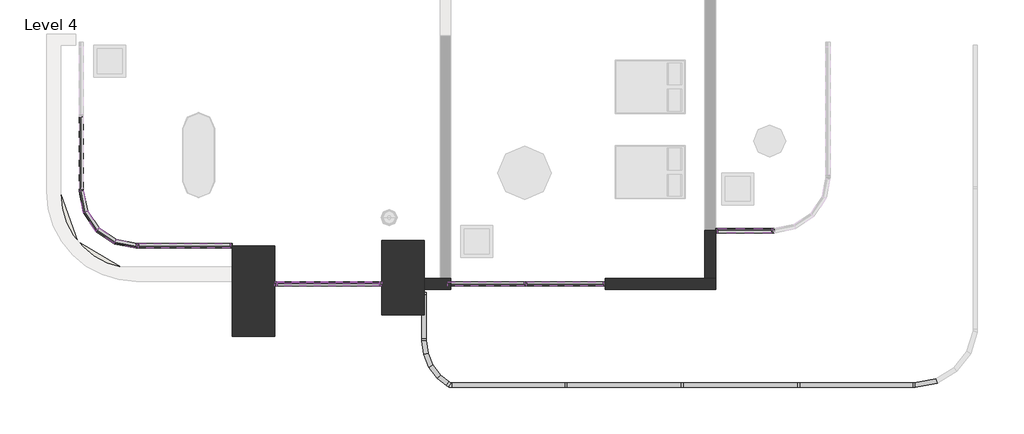
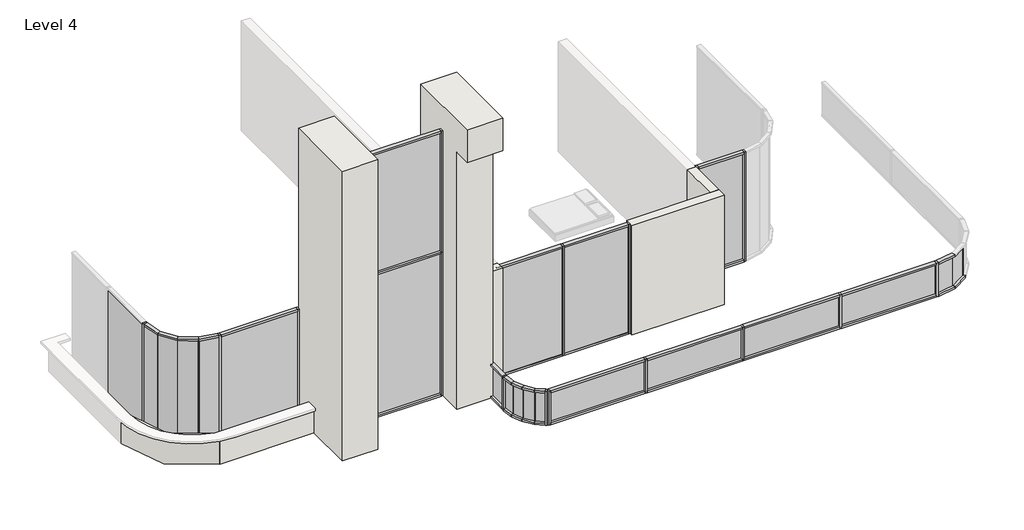
# One storey, part 1 of 2: 61 members, 22 plates, 7 walls.
"""IFC4 building model written with IfcOpenShell, lengths in millimetres."""

from ifc_helpers import new_model, si_unit, point, frame, frame_2d, origin, place, context, project, spatial, polyline, circle_curve, trimmed, segment, composite_curve, outline, extrude, faceted_brep, transform, mapped, element, save
from components import member_e5c989f4, member_5be86ab4, member_8daf8b49, member_d457d5cf, member_70c1698b, member_c6c1cc64, member_2ed7bf35, member_fedd83b6, member_820ab859, member_e6e8f276, member_9bbfae49, member_71eb4692, member_3c8bcf7e, member_dede372a, member_2b49869a, member_75074519, member_068c4367, member_d18c953d, member_1e511d5c, member_f1972444, member_37af120a, member_fe018dc2, member_83685764, member_73d0c9ee, member_70a47126, member_8f078878, system_panel_glazed_da3fd9d5, system_panel_glazed_e9252991, system_panel_glazed_d7bd2e6f, system_panel_glazed_62c681ce, system_panel_glazed_5d8041e7, system_panel_glazed_8818662e, system_panel_glazed_df7f3c5e, system_panel_glazed_53e0be6b, system_panel_glazed_e0d10779, system_panel_glazed_9262d402, system_panel_glazed_b9e36109, system_panel_glazed_ffaa535b, system_panel_glazed_1f819173

model = new_model("IFC4")

# Units and contexts
model_context = context("Model", 3, world=origin())
ifc_project = project(units=[si_unit("LENGTHUNIT", "METRE", prefix="MILLI")], contexts=[model_context])

# Site, building, storey
site = spatial("IfcSite", under=ifc_project)
building = spatial("IfcBuilding", under=site)
storey = spatial("IfcBuildingStorey", under=building, Name="Level 4", Elevation=6096.0)

# Members
placement = place(None, origin())
member_shape = member_e5c989f4(model_context)
element("IfcMember", 1, ObjectType="Rectangular Mullion : 2.5\" x 5\" rectangular", at=placement, inside=storey, context=model_context, shape_type="MappedRepresentation", body=[
    mapped(member_shape, transform((-4022.036879, -4118.7908042, 5994.4), x_axis=(-1.0, 0.0, 0.0), y_axis=(0.0, 1.0, 0.0), z_axis=(0.0, 0.0, -1.0))),
])
member_2_shape = member_5be86ab4(model_context)
element("IfcMember", 2, ObjectType="Rectangular Mullion : 2.5\" x 5\" rectangular", at=placement, inside=storey, context=model_context, shape_type="MappedRepresentation", body=[
    mapped(member_2_shape, transform((-6308.036879, -4118.7908042, 5994.4), x_axis=(-1.0, 0.0, 0.0), y_axis=(0.0, 1.0, 0.0), z_axis=(0.0, 0.0, -1.0))),
])
element("IfcMember", 3, ObjectType="Rectangular Mullion : 2.5\" x 5\" rectangular", at=placement, inside=storey, context=model_context, shape_type="MappedRepresentation", body=[
    mapped(member_2_shape, transform((3089.963121, -2594.7908042, 5994.4), x_axis=(1.0, 0.0, 0.0), y_axis=(0.0, -1.0, 0.0), z_axis=(0.0, 0.0, -1.0))),
])
element("IfcMember", 4, ObjectType="Rectangular Mullion : 2.5\" x 5\" rectangular", at=placement, inside=storey, context=model_context, shape_type="MappedRepresentation", body=[
    mapped(member_2_shape, transform((-15147.236879, -3028.3602909, 5994.4), x_axis=(-1.0, 0.0, 0.0), y_axis=(0.0, 1.0, 0.0), z_axis=(0.0, 0.0, -1.0))),
])
element("IfcMember", 5, ObjectType="Rectangular Mullion : 2.5\" x 5\" rectangular", at=placement, inside=storey, context=model_context, shape_type="MappedRepresentation", body=[
    mapped(member_2_shape, transform((-1736.036879, -4118.7908042, 9956.8), x_axis=(1.0, 0.0, 0.0), y_axis=(0.0, 1.0, 0.0), z_axis=(0.0, 0.0, 1.0))),
])
element("IfcMember", 6, ObjectType="Rectangular Mullion : 2.5\" x 5\" rectangular", at=placement, inside=storey, context=model_context, shape_type="MappedRepresentation", body=[
    mapped(member_2_shape, transform((1413.563121, -2594.7908042, 9956.8), x_axis=(-1.0, 0.0, 0.0), y_axis=(0.0, -1.0, 0.0), z_axis=(0.0, 0.0, 1.0))),
])
element("IfcMember", 7, ObjectType="Rectangular Mullion : 2.5\" x 5\" rectangular", at=placement, inside=storey, context=model_context, shape_type="MappedRepresentation", body=[
    mapped(member_2_shape, transform((-12404.036879, -3028.3602909, 9956.8), x_axis=(1.0, 0.0, 0.0), y_axis=(0.0, 1.0, 0.0), z_axis=(0.0, 0.0, 1.0))),
])
element("IfcMember", 8, ObjectType="Rectangular Mullion : 2.5\" x 5\" rectangular", at=placement, inside=storey, context=model_context, shape_type="MappedRepresentation", body=[
    mapped(member_2_shape, transform((-16724.4155088, -1451.181661, 9956.8), x_axis=(0.0, -1.0, 0.0), y_axis=(1.0, 0.0, 0.0), z_axis=(0.0, 0.0, 1.0))),
])
member_3_shape = member_8daf8b49(model_context)
element("IfcMember", 9, ObjectType="Rectangular Mullion : 2.5\" x 5\" rectangular", at=placement, inside=storey, context=model_context, shape_type="MappedRepresentation", body=[
    mapped(member_3_shape, transform((-6244.536879, -4118.7908042, 9956.8), x_axis=(0.0, 0.0, 1.0), y_axis=(0.0, 1.0, 0.0), z_axis=(-1.0, 0.0, 0.0))),
])
element("IfcMember", 10, ObjectType="Rectangular Mullion : 2.5\" x 5\" rectangular", at=placement, inside=storey, context=model_context, shape_type="MappedRepresentation", body=[
    mapped(member_3_shape, transform((-3990.286879, -4118.7908042, 9956.8), x_axis=(0.0, 0.0, 1.0), y_axis=(0.0, 1.0, 0.0), z_axis=(-1.0, 0.0, 0.0))),
])
element("IfcMember", 11, ObjectType="Rectangular Mullion : 2.5\" x 5\" rectangular", at=placement, inside=storey, context=model_context, shape_type="MappedRepresentation", body=[
    mapped(member_3_shape, transform((-1799.536879, -4118.7908042, 5994.4), x_axis=(0.0, 0.0, -1.0), y_axis=(0.0, 1.0, 0.0), z_axis=(1.0, 0.0, 0.0))),
])
element("IfcMember", 12, ObjectType="Rectangular Mullion : 2.5\" x 5\" rectangular", at=placement, inside=storey, context=model_context, shape_type="MappedRepresentation", body=[
    mapped(member_3_shape, transform((-4053.786879, -4118.7908042, 5994.4), x_axis=(0.0, 0.0, -1.0), y_axis=(0.0, 1.0, 0.0), z_axis=(1.0, 0.0, 0.0))),
])
member_4_shape = member_d457d5cf(model_context)
element("IfcMember", 13, ObjectType="Rectangular Mullion : 2.5\" x 5\" rectangular", at=placement, inside=storey, context=model_context, shape_type="MappedRepresentation", body=[
    mapped(member_4_shape, transform((-8200.336879, -4118.7908042, 15572.5549749), x_axis=(0.0, 0.0, 1.0), y_axis=(0.0, -1.0, 0.0), z_axis=(1.0, 0.0, 0.0))),
])
element("IfcMember", 14, ObjectType="Rectangular Mullion : 2.5\" x 5\" rectangular", at=placement, inside=storey, context=model_context, shape_type="MappedRepresentation", body=[
    mapped(member_4_shape, transform((-11121.336879, -4118.7908042, 5994.4), x_axis=(0.0, 0.0, -1.0), y_axis=(0.0, -1.0, 0.0), z_axis=(-1.0, 0.0, 0.0))),
])
member_5_shape = member_70c1698b(model_context)
element("IfcMember", 15, ObjectType="Rectangular Mullion : 2.5\" x 5\" rectangular", at=placement, inside=storey, context=model_context, shape_type="MappedRepresentation", body=[
    mapped(member_5_shape, transform((-15083.736879, -3028.3602909, 9956.8), x_axis=(0.0, 0.0, 1.0), y_axis=(0.0, 1.0, 0.0), z_axis=(-1.0, 0.0, 0.0))),
])
element("IfcMember", 16, ObjectType="Rectangular Mullion : 2.5\" x 5\" rectangular", at=placement, inside=storey, context=model_context, shape_type="MappedRepresentation", body=[
    mapped(member_5_shape, transform((-12467.536879, -3028.3602909, 5994.4), x_axis=(0.0, 0.0, -1.0), y_axis=(0.0, 1.0, 0.0), z_axis=(1.0, 0.0, 0.0))),
])
member_6_shape = member_c6c1cc64(model_context)
element("IfcMember", 17, ObjectType="Rectangular Mullion : 2.5\" x 5\" rectangular", at=placement, inside=storey, context=model_context, shape_type="MappedRepresentation", body=[
    mapped(member_6_shape, transform((-16262.4705833, -2566.4153653, 9956.8), x_axis=(0.0, 0.0, 1.0), y_axis=(0.5555702330196196, 0.8314696123025338, 0.0), z_axis=(-0.8314696123025338, 0.5555702330196196, 0.0))),
])
element("IfcMember", 18, ObjectType="Rectangular Mullion : 2.5\" x 5\" rectangular", at=placement, inside=storey, context=model_context, shape_type="MappedRepresentation", body=[
    mapped(member_6_shape, transform((-15750.7970105, -2908.3047162, 5994.4), x_axis=(0.0, 0.0, -1.0), y_axis=(0.5555702330196196, 0.8314696123025338, 0.0), z_axis=(0.8314696123025338, -0.5555702330196196, 0.0))),
])
element("IfcMember", 19, ObjectType="Rectangular Mullion : 2.5\" x 5\" rectangular", at=placement, inside=storey, context=model_context, shape_type="MappedRepresentation", body=[
    mapped(member_6_shape, transform((-16262.4705833, -2566.4153653, 5994.4), x_axis=(0.0, 0.0, -1.0), y_axis=(0.831469612302556, 0.5555702330195863, 0.0), z_axis=(0.5555702330195863, -0.831469612302556, 0.0))),
])
element("IfcMember", 20, ObjectType="Rectangular Mullion : 2.5\" x 5\" rectangular", at=placement, inside=storey, context=model_context, shape_type="MappedRepresentation", body=[
    mapped(member_6_shape, transform((-16604.3599342, -2054.7417925, 9956.8), x_axis=(0.0, 0.0, 1.0), y_axis=(0.8314696123025557, 0.5555702330195866, 0.0), z_axis=(-0.5555702330195866, 0.8314696123025557, 0.0))),
])
member_7_shape = member_2ed7bf35(model_context)
element("IfcMember", 21, ObjectType="Rectangular Mullion : 2.5\" x 5\" rectangular", at=placement, inside=storey, context=model_context, shape_type="MappedRepresentation", body=[
    mapped(member_7_shape, transform((-8200.336879, -4118.7908042, 11176.0), x_axis=(0.0, 0.0, 1.0), y_axis=(0.0, -1.0, 0.0), z_axis=(1.0, 0.0, 0.0))),
])
member_8_shape = member_fedd83b6(model_context)
element("IfcMember", 22, ObjectType="Rectangular Mullion : 2.5\" x 5\" rectangular", at=placement, inside=storey, context=model_context, shape_type="MappedRepresentation", body=[
    mapped(member_8_shape, transform((3026.463121, -2594.7908042, 9956.8), x_axis=(0.0, 0.0, 1.0), y_axis=(0.0, -1.0, 0.0), z_axis=(1.0, 0.0, 0.0))),
])
element("IfcMember", 23, ObjectType="Rectangular Mullion : 2.5\" x 5\" rectangular", at=placement, inside=storey, context=model_context, shape_type="MappedRepresentation", body=[
    mapped(member_8_shape, transform((1477.063121, -2594.7908042, 5994.4), x_axis=(0.0, 0.0, -1.0), y_axis=(0.0, -1.0, 0.0), z_axis=(-1.0, 0.0, 0.0))),
])
member_9_shape = member_820ab859(model_context)
element("IfcMember", 24, ObjectType="Rectangular Mullion : 2.5\" x 5\" rectangular", at=placement, inside=storey, context=model_context, shape_type="MappedRepresentation", body=[
    mapped(member_9_shape, transform((-16724.4155088, -1387.681661, 5994.4), x_axis=(0.0, 0.0, -1.0), y_axis=(1.0, 0.0, 0.0), z_axis=(0.0, -1.0, 0.0))),
])
member_10_shape = member_e6e8f276(model_context)
element("IfcMember", 25, ObjectType="Rectangular Mullion : 2.5\" x 5\" rectangular", at=placement, inside=storey, context=model_context, shape_type="MappedRepresentation", body=[
    mapped(member_10_shape, transform((-15147.236879, -3028.3602909, 5994.4), x_axis=(0.0, 0.0, -1.0), y_axis=(0.19509032201614443, 0.9807852804032272, 0.0), z_axis=(0.9807852804032271, -0.1950903220161444, 0.0))),
])
member_11_shape = member_9bbfae49(model_context)
element("IfcMember", 26, ObjectType="Rectangular Mullion : 2.5\" x 5\" rectangular", at=placement, inside=storey, context=model_context, shape_type="MappedRepresentation", body=[
    mapped(member_11_shape, transform((-15750.7970105, -2908.3047162, 9956.8), x_axis=(0.0, 0.0, 1.0), y_axis=(0.19509032201614443, 0.9807852804032272, 0.0), z_axis=(-0.9807852804032271, 0.1950903220161444, 0.0))),
])
element("IfcMember", 27, ObjectType="Rectangular Mullion : 2.5\" x 5\" rectangular", at=placement, inside=storey, context=model_context, shape_type="MappedRepresentation", body=[
    mapped(member_10_shape, transform((-16724.4155088, -1451.181661, 9956.8), x_axis=(0.0, 0.0, 1.0), y_axis=(0.9807852804032322, 0.1950903220161199, 0.0), z_axis=(-0.1950903220161199, 0.9807852804032322, 0.0))),
])
element("IfcMember", 28, ObjectType="Rectangular Mullion : 2.5\" x 5\" rectangular", at=placement, inside=storey, context=model_context, shape_type="MappedRepresentation", body=[
    mapped(member_11_shape, transform((-16604.3599342, -2054.7417925, 5994.4), x_axis=(0.0, 0.0, -1.0), y_axis=(0.9807852804032322, 0.1950903220161199, 0.0), z_axis=(0.1950903220161199, -0.9807852804032322, 0.0))),
])
member_12_shape = member_71eb4692(model_context)
element("IfcMember", 29, ObjectType="Rectangular Mullion : 2.5\" x 5\" rectangular", at=placement, inside=storey, context=model_context, shape_type="MappedRepresentation", body=[
    mapped(member_12_shape, transform((-6917.636879, -5676.9, 7213.6), x_axis=(0.0, 0.0, 1.0), y_axis=(-1.0, 0.0, 0.0), z_axis=(0.0, -1.0, 0.0))),
])
element("IfcMember", 30, ObjectType="Rectangular Mullion : 2.5\" x 5\" rectangular", at=placement, inside=storey, context=model_context, shape_type="MappedRepresentation", body=[
    mapped(member_12_shape, transform((-6917.636879, -4432.3, 5994.4), x_axis=(0.0, 0.0, -1.0), y_axis=(-1.0, 0.0, 0.0), z_axis=(0.0, 1.0, 0.0))),
])
member_13_shape = member_3c8bcf7e(model_context)
element("IfcMember", 31, ObjectType="Rectangular Mullion : 2.5\" x 5\" rectangular", at=placement, inside=storey, context=model_context, shape_type="MappedRepresentation", body=[
    mapped(member_13_shape, transform((7048.5, -7010.4, 7213.6), x_axis=(0.0, 0.0, 1.0), y_axis=(0.0, -1.0, 0.0), z_axis=(1.0, 0.0, 0.0))),
])
element("IfcMember", 32, ObjectType="Rectangular Mullion : 2.5\" x 5\" rectangular", at=placement, inside=storey, context=model_context, shape_type="MappedRepresentation", body=[
    mapped(member_13_shape, transform((-2901.95, -7010.4, 7213.6), x_axis=(0.0, 0.0, 1.0), y_axis=(0.0, -1.0, 0.0), z_axis=(1.0, 0.0, 0.0))),
])
member_14_shape = member_dede372a(model_context)
element("IfcMember", 33, ObjectType="Rectangular Mullion : 2.5\" x 5\" rectangular", at=placement, inside=storey, context=model_context, shape_type="MappedRepresentation", body=[
    mapped(member_14_shape, transform((425.45, -7010.4, 7213.6), x_axis=(0.0, 0.0, 1.0), y_axis=(0.0, -1.0, 0.0), z_axis=(1.0, 0.0, 0.0))),
])
element("IfcMember", 34, ObjectType="Rectangular Mullion : 2.5\" x 5\" rectangular", at=placement, inside=storey, context=model_context, shape_type="MappedRepresentation", body=[
    mapped(member_14_shape, transform((3752.85, -7010.4, 7213.6), x_axis=(0.0, 0.0, 1.0), y_axis=(0.0, -1.0, 0.0), z_axis=(1.0, 0.0, 0.0))),
])
element("IfcMember", 35, ObjectType="Rectangular Mullion : 2.5\" x 5\" rectangular", at=placement, inside=storey, context=model_context, shape_type="MappedRepresentation", body=[
    mapped(member_13_shape, transform((-6134.1, -7010.4, 5994.4), x_axis=(0.0, 0.0, -1.0), y_axis=(0.0, -1.0, 0.0), z_axis=(-1.0, 0.0, 0.0))),
])
element("IfcMember", 36, ObjectType="Rectangular Mullion : 2.5\" x 5\" rectangular", at=placement, inside=storey, context=model_context, shape_type="MappedRepresentation", body=[
    mapped(member_13_shape, transform((3816.35, -7010.4, 5994.4), x_axis=(0.0, 0.0, -1.0), y_axis=(0.0, -1.0, 0.0), z_axis=(-1.0, 0.0, 0.0))),
])
element("IfcMember", 37, ObjectType="Rectangular Mullion : 2.5\" x 5\" rectangular", at=placement, inside=storey, context=model_context, shape_type="MappedRepresentation", body=[
    mapped(member_14_shape, transform((-2838.45, -7010.4, 5994.4), x_axis=(0.0, 0.0, -1.0), y_axis=(0.0, -1.0, 0.0), z_axis=(-1.0, 0.0, 0.0))),
])
element("IfcMember", 38, ObjectType="Rectangular Mullion : 2.5\" x 5\" rectangular", at=placement, inside=storey, context=model_context, shape_type="MappedRepresentation", body=[
    mapped(member_14_shape, transform((488.95, -7010.4, 5994.4), x_axis=(0.0, 0.0, -1.0), y_axis=(0.0, -1.0, 0.0), z_axis=(-1.0, 0.0, 0.0))),
])
member_15_shape = member_2b49869a(model_context)
element("IfcMember", 39, ObjectType="Rectangular Mullion : 2.5\" x 5\" rectangular", at=placement, inside=storey, context=model_context, shape_type="MappedRepresentation", body=[
    mapped(member_15_shape, transform((-2870.2, -7010.4, 5994.4), x_axis=(1.0, 0.0, 0.0), y_axis=(0.0, -1.0, 0.0), z_axis=(0.0, 0.0, -1.0))),
])
element("IfcMember", 40, ObjectType="Rectangular Mullion : 2.5\" x 5\" rectangular", at=placement, inside=storey, context=model_context, shape_type="MappedRepresentation", body=[
    mapped(member_15_shape, transform((457.2, -7010.4, 5994.4), x_axis=(1.0, 0.0, 0.0), y_axis=(0.0, -1.0, 0.0), z_axis=(0.0, 0.0, -1.0))),
])
element("IfcMember", 41, ObjectType="Rectangular Mullion : 2.5\" x 5\" rectangular", at=placement, inside=storey, context=model_context, shape_type="MappedRepresentation", body=[
    mapped(member_15_shape, transform((3784.6, -7010.4, 5994.4), x_axis=(1.0, 0.0, 0.0), y_axis=(0.0, -1.0, 0.0), z_axis=(0.0, 0.0, -1.0))),
])
member_16_shape = member_75074519(model_context)
element("IfcMember", 42, ObjectType="Rectangular Mullion : 2.5\" x 5\" rectangular", at=placement, inside=storey, context=model_context, shape_type="MappedRepresentation", body=[
    mapped(member_16_shape, transform((-6917.636879, -5740.4, 5994.4), x_axis=(0.0, -1.0, 0.0), y_axis=(-1.0, 0.0, 0.0), z_axis=(0.0, 0.0, -1.0))),
])
element("IfcMember", 43, ObjectType="Rectangular Mullion : 2.5\" x 5\" rectangular", at=placement, inside=storey, context=model_context, shape_type="MappedRepresentation", body=[
    mapped(member_16_shape, transform((-6197.6, -7010.4, 5994.4), x_axis=(0.7849384979521701, -0.6195736876535278, 0.0), y_axis=(-0.6195736876535278, -0.7849384979521701, 0.0), z_axis=(0.0, 0.0, -1.0))),
])
element("IfcMember", 44, ObjectType="Rectangular Mullion : 2.5\" x 5\" rectangular", at=placement, inside=storey, context=model_context, shape_type="MappedRepresentation", body=[
    mapped(member_16_shape, transform((7112.0, -7010.4, 5994.4), x_axis=(1.0, 0.0, 0.0), y_axis=(0.0, -1.0, 0.0), z_axis=(0.0, 0.0, -1.0))),
])
element("IfcMember", 45, ObjectType="Rectangular Mullion : 2.5\" x 5\" rectangular", at=placement, inside=storey, context=model_context, shape_type="MappedRepresentation", body=[
    mapped(member_16_shape, transform((-6917.636879, -4368.8, 7213.6), x_axis=(0.0, 1.0, 0.0), y_axis=(-1.0, 0.0, 0.0), z_axis=(0.0, 0.0, 1.0))),
])
element("IfcMember", 46, ObjectType="Rectangular Mullion : 2.5\" x 5\" rectangular", at=placement, inside=storey, context=model_context, shape_type="MappedRepresentation", body=[
    mapped(member_16_shape, transform((-6197.6, -7010.4, 7213.6), x_axis=(-1.0, 0.0, 0.0), y_axis=(0.0, -1.0, 0.0), z_axis=(0.0, 0.0, 1.0))),
])
member_17_shape = member_068c4367(model_context)
element("IfcMember", 47, ObjectType="Rectangular Mullion : 2.5\" x 5\" rectangular", at=placement, inside=storey, context=model_context, shape_type="MappedRepresentation", body=[
    mapped(member_17_shape, transform((-6247.4435946, -6971.0570708, 7213.6), x_axis=(0.0, 0.0, 1.0), y_axis=(-0.6195736876535282, -0.7849384979521697, 0.0), z_axis=(0.7849384979521697, -0.6195736876535282, 0.0))),
])
member_18_shape = member_d18c953d(model_context)
element("IfcMember", 48, ObjectType="Rectangular Mullion : 2.5\" x 5\" rectangular", at=placement, inside=storey, context=model_context, shape_type="MappedRepresentation", body=[
    mapped(member_18_shape, transform((-6496.3637925, -6774.5774672, 5994.4), x_axis=(0.0, 0.0, -1.0), y_axis=(-0.6195736876535282, -0.7849384979521697, 0.0), z_axis=(-0.7849384979521697, 0.6195736876535282, 0.0))),
])
member_19_shape = member_1e511d5c(model_context)
element("IfcMember", 49, ObjectType="Rectangular Mullion : 2.5\" x 5\" rectangular", at=placement, inside=storey, context=model_context, shape_type="MappedRepresentation", body=[
    mapped(member_19_shape, transform((-6725.1047325, -6470.3577226, 5994.4), x_axis=(0.0, 0.0, -1.0), y_axis=(-0.7992728550453325, -0.6009683046448315, 0.0), z_axis=(-0.6009683046448315, 0.7992728550453325, 0.0))),
])
element("IfcMember", 50, ObjectType="Rectangular Mullion : 2.5\" x 5\" rectangular", at=placement, inside=storey, context=model_context, shape_type="MappedRepresentation", body=[
    mapped(member_19_shape, transform((-6496.3637925, -6774.5774672, 7213.6), x_axis=(0.0, 0.0, 1.0), y_axis=(-0.7992728550453325, -0.6009683046448315, 0.0), z_axis=(0.6009683046448315, -0.7992728550453325, 0.0))),
])
element("IfcMember", 51, ObjectType="Rectangular Mullion : 2.5\" x 5\" rectangular", at=placement, inside=storey, context=model_context, shape_type="MappedRepresentation", body=[
    mapped(member_19_shape, transform((-6725.1047325, -6470.3577226, 7213.6), x_axis=(0.0, 0.0, 1.0), y_axis=(-0.9261106552646661, -0.3772519770726865, 0.0), z_axis=(0.3772519770726865, -0.9261106552646661, 0.0))),
])
element("IfcMember", 52, ObjectType="Rectangular Mullion : 2.5\" x 5\" rectangular", at=placement, inside=storey, context=model_context, shape_type="MappedRepresentation", body=[
    mapped(member_19_shape, transform((-6868.694621, -6117.8608934, 5994.4), x_axis=(0.0, 0.0, -1.0), y_axis=(-0.9261106552646661, -0.3772519770726865, 0.0), z_axis=(-0.3772519770726865, 0.9261106552646661, 0.0))),
])
member_20_shape = member_f1972444(model_context)
element("IfcMember", 53, ObjectType="Rectangular Mullion : 2.5\" x 5\" rectangular", at=placement, inside=storey, context=model_context, shape_type="MappedRepresentation", body=[
    mapped(member_20_shape, transform((-6917.636879, -5740.4, 5994.4), x_axis=(0.0, 0.0, -1.0), y_axis=(-0.9916984391957502, -0.12858540234689558, 0.0), z_axis=(-0.12858540234689556, 0.9916984391957501, 0.0))),
])
member_21_shape = member_37af120a(model_context)
element("IfcMember", 54, ObjectType="Rectangular Mullion : 2.5\" x 5\" rectangular", at=placement, inside=storey, context=model_context, shape_type="MappedRepresentation", body=[
    mapped(member_21_shape, transform((-6868.694621, -6117.8608934, 7213.6), x_axis=(0.0, 0.0, 1.0), y_axis=(-0.9916984391957502, -0.12858540234689558, 0.0), z_axis=(0.12858540234689556, -0.9916984391957501, 0.0))),
])
member_22_shape = member_fe018dc2(model_context)
element("IfcMember", 55, ObjectType="Rectangular Mullion : 2.5\" x 5\" rectangular", at=placement, inside=storey, context=model_context, shape_type="MappedRepresentation", body=[
    mapped(member_22_shape, transform((7727.6464366, -6897.8973023, 5994.4), x_axis=(0.0, 0.0, -1.0), y_axis=(0.5160512694614303, -0.8565576964146936, 0.0), z_axis=(-0.8565576964146935, -0.5160512694614302, 0.0))),
])
member_23_shape = member_83685764(model_context)
element("IfcMember", 56, ObjectType="Rectangular Mullion : 2.5\" x 5\" rectangular", at=placement, inside=storey, context=model_context, shape_type="MappedRepresentation", body=[
    mapped(member_23_shape, transform((7112.0, -7010.4, 5994.4), x_axis=(0.0, 0.0, -1.0), y_axis=(0.1797623282098431, -0.9837100717978732, 0.0), z_axis=(-0.9837100717978732, -0.1797623282098431, 0.0))),
])
member_24_shape = member_73d0c9ee(model_context)
element("IfcMember", 57, ObjectType="Rectangular Mullion : 2.5\" x 5\" rectangular", at=placement, inside=storey, context=model_context, shape_type="MappedRepresentation", body=[
    mapped(member_24_shape, transform((7727.6464366, -6897.8973023, 7213.6), x_axis=(0.0, 0.0, 1.0), y_axis=(0.1797623282098431, -0.9837100717978732, 0.0), z_axis=(0.9837100717978732, 0.1797623282098431, 0.0))),
])
member_25_shape = member_70a47126(model_context)
element("IfcMember", 58, ObjectType="Rectangular Mullion : 2.5\" x 5\" rectangular", at=placement, inside=storey, context=model_context, shape_type="MappedRepresentation", body=[
    mapped(member_25_shape, transform((-8136.836879, -4118.7908042, 5994.4), x_axis=(1.0, 0.0, 0.0), y_axis=(0.0, -1.0, 0.0), z_axis=(0.0, 0.0, -1.0))),
])
element("IfcMember", 59, ObjectType="Rectangular Mullion : 2.5\" x 5\" rectangular", at=placement, inside=storey, context=model_context, shape_type="MappedRepresentation", body=[
    mapped(member_25_shape, transform((-11184.836879, -4118.7908042, 11176.0), x_axis=(-1.0, 0.0, 0.0), y_axis=(0.0, -1.0, 0.0), z_axis=(0.0, 0.0, 1.0))),
])
member_26_shape = member_8f078878(model_context)
element("IfcMember", 60, ObjectType="Rectangular Mullion : 2.5\" x 5\" rectangular", at=placement, inside=storey, context=model_context, shape_type="MappedRepresentation", body=[
    mapped(member_26_shape, transform((-11184.836879, -4118.7908042, 15572.5549749), x_axis=(-1.0, 0.0, 0.0), y_axis=(0.0, -1.0, 0.0), z_axis=(0.0, 0.0, 1.0))),
])
element("IfcMember", 61, ObjectType="Rectangular Mullion : 2.5\" x 5\" rectangular", at=placement, inside=storey, context=model_context, shape_type="MappedRepresentation", body=[
    mapped(member_26_shape, transform((-8136.836879, -4118.7908042, 11176.0), x_axis=(1.0, 0.0, 0.0), y_axis=(0.0, -1.0, 0.0), z_axis=(0.0, 0.0, -1.0))),
])

# Plates
system_panel_glazed_shape = system_panel_glazed_da3fd9d5(model_context)
element("IfcPlate", 62, ObjectType="System Panel : Glazed", at=placement, inside=storey, context=model_context, shape_type="MappedRepresentation", body=[
    mapped(system_panel_glazed_shape, transform((-2894.911879, -4118.7908042, 6057.9), x_axis=(-1.0, 0.0, 0.0), y_axis=(0.0, -1.0, 0.0), z_axis=(0.0, 0.0, 1.0))),
])
element("IfcPlate", 63, ObjectType="System Panel : Glazed", at=placement, inside=storey, context=model_context, shape_type="MappedRepresentation", body=[
    mapped(system_panel_glazed_shape, transform((-5149.161879, -4118.7908042, 6057.9), x_axis=(-1.0, 0.0, 0.0), y_axis=(0.0, -1.0, 0.0), z_axis=(0.0, 0.0, 1.0))),
])
system_panel_glazed_2_shape = system_panel_glazed_e9252991(model_context)
element("IfcPlate", 64, ObjectType="System Panel : Glazed", at=placement, inside=storey, context=model_context, shape_type="MappedRepresentation", body=[
    mapped(system_panel_glazed_2_shape, transform((-13775.636879, -3028.3602909, 6057.9), x_axis=(-1.0, 0.0, 0.0), y_axis=(0.0, -1.0, 0.0), z_axis=(0.0, 0.0, 1.0))),
])
system_panel_glazed_3_shape = system_panel_glazed_d7bd2e6f(model_context)
element("IfcPlate", 65, ObjectType="System Panel : Glazed", at=placement, inside=storey, context=model_context, shape_type="MappedRepresentation", body=[
    mapped(system_panel_glazed_3_shape, transform((-15449.0169447, -2968.3325036, 6057.9), x_axis=(-0.9807852804032273, 0.19509032201614446, 0.0), y_axis=(-0.19509032201614446, -0.9807852804032273, 0.0), z_axis=(0.0, 0.0, 1.0))),
])
element("IfcPlate", 66, ObjectType="System Panel : Glazed", at=placement, inside=storey, context=model_context, shape_type="MappedRepresentation", body=[
    mapped(system_panel_glazed_3_shape, transform((-16433.4152587, -2310.5785789, 6057.9), x_axis=(-0.5555702330195869, 0.8314696123025556, 0.0), y_axis=(-0.8314696123025556, -0.5555702330195869, 0.0), z_axis=(0.0, 0.0, 1.0))),
])
element("IfcPlate", 67, ObjectType="System Panel : Glazed", at=placement, inside=storey, context=model_context, shape_type="MappedRepresentation", body=[
    mapped(system_panel_glazed_3_shape, transform((-16664.3877215, -1752.9617268, 6057.9), x_axis=(-0.1950903220161199, 0.9807852804032322, 0.0), y_axis=(-0.9807852804032322, -0.1950903220161199, 0.0), z_axis=(0.0, 0.0, 1.0))),
])
element("IfcPlate", 68, ObjectType="System Panel : Glazed", at=placement, inside=storey, context=model_context, shape_type="MappedRepresentation", body=[
    mapped(system_panel_glazed_3_shape, transform((-16006.6337969, -2737.3600408, 6057.9), x_axis=(-0.8314696123025338, 0.5555702330196196, 0.0), y_axis=(-0.5555702330196196, -0.8314696123025338, 0.0), z_axis=(0.0, 0.0, 1.0))),
])
system_panel_glazed_4_shape = system_panel_glazed_62c681ce(model_context)
element("IfcPlate", 69, ObjectType="System Panel : Glazed", at=placement, inside=storey, context=model_context, shape_type="MappedRepresentation", body=[
    mapped(system_panel_glazed_4_shape, transform((2251.763121, -2594.7908042, 6057.9), x_axis=(1.0, 0.0, 0.0), y_axis=(0.0, 1.0, 0.0), z_axis=(0.0, 0.0, 1.0))),
])
system_panel_glazed_5_shape = system_panel_glazed_5d8041e7(model_context)
element("IfcPlate", 70, ObjectType="System Panel : Glazed", at=placement, inside=storey, context=model_context, shape_type="MappedRepresentation", body=[
    mapped(system_panel_glazed_5_shape, transform((-16724.4155088, -354.8003023, 6057.9), x_axis=(0.0, 1.0, 0.0), y_axis=(-1.0, 0.0, 0.0), z_axis=(0.0, 0.0, 1.0))),
])
system_panel_glazed_6_shape = system_panel_glazed_8818662e(model_context)
element("IfcPlate", 71, ObjectType="System Panel : Glazed", at=placement, inside=storey, context=model_context, shape_type="MappedRepresentation", body=[
    mapped(system_panel_glazed_6_shape, transform((-4518.025, -7010.4, 6057.9), x_axis=(1.0, 0.0, 0.0), y_axis=(0.0, 1.0, 0.0), z_axis=(0.0, 0.0, 1.0))),
])
element("IfcPlate", 72, ObjectType="System Panel : Glazed", at=placement, inside=storey, context=model_context, shape_type="MappedRepresentation", body=[
    mapped(system_panel_glazed_6_shape, transform((5432.425, -7010.4, 6057.9), x_axis=(1.0, 0.0, 0.0), y_axis=(0.0, 1.0, 0.0), z_axis=(0.0, 0.0, 1.0))),
])
system_panel_glazed_7_shape = system_panel_glazed_df7f3c5e(model_context)
element("IfcPlate", 73, ObjectType="System Panel : Glazed", at=placement, inside=storey, context=model_context, shape_type="MappedRepresentation", body=[
    mapped(system_panel_glazed_7_shape, transform((-1206.5, -7010.4, 6057.9), x_axis=(1.0, 0.0, 0.0), y_axis=(0.0, 1.0, 0.0), z_axis=(0.0, 0.0, 1.0))),
])
element("IfcPlate", 74, ObjectType="System Panel : Glazed", at=placement, inside=storey, context=model_context, shape_type="MappedRepresentation", body=[
    mapped(system_panel_glazed_7_shape, transform((2120.9, -7010.4, 6057.9), x_axis=(1.0, 0.0, 0.0), y_axis=(0.0, 1.0, 0.0), z_axis=(0.0, 0.0, 1.0))),
])
system_panel_glazed_8_shape = system_panel_glazed_53e0be6b(model_context)
element("IfcPlate", 75, ObjectType="System Panel : Glazed", at=placement, inside=storey, context=model_context, shape_type="MappedRepresentation", body=[
    mapped(system_panel_glazed_8_shape, transform((-6917.636879, -5054.6, 6057.9), x_axis=(0.0, -1.0, 0.0), y_axis=(1.0, 0.0, 0.0), z_axis=(0.0, 0.0, 1.0))),
])
system_panel_glazed_9_shape = system_panel_glazed_e0d10779(model_context)
element("IfcPlate", 76, ObjectType="System Panel : Glazed", at=placement, inside=storey, context=model_context, shape_type="MappedRepresentation", body=[
    mapped(system_panel_glazed_9_shape, transform((-6371.9036936, -6872.817269, 6057.9), x_axis=(0.7849384979521701, -0.6195736876535278, 0.0), y_axis=(0.6195736876535278, 0.7849384979521701, 0.0), z_axis=(0.0, 0.0, 1.0))),
])
system_panel_glazed_10_shape = system_panel_glazed_9262d402(model_context)
element("IfcPlate", 77, ObjectType="System Panel : Glazed", at=placement, inside=storey, context=model_context, shape_type="MappedRepresentation", body=[
    mapped(system_panel_glazed_10_shape, transform((-6893.16575, -5929.1304467, 6057.9), x_axis=(0.12858540234689558, -0.9916984391957502, 0.0), y_axis=(0.9916984391957502, 0.12858540234689558, 0.0), z_axis=(0.0, 0.0, 1.0))),
])
element("IfcPlate", 78, ObjectType="System Panel : Glazed", at=placement, inside=storey, context=model_context, shape_type="MappedRepresentation", body=[
    mapped(system_panel_glazed_10_shape, transform((-6610.7342625, -6622.4675949, 6057.9), x_axis=(0.6009683046448315, -0.7992728550453325, 0.0), y_axis=(0.7992728550453325, 0.6009683046448315, 0.0), z_axis=(0.0, 0.0, 1.0))),
])
element("IfcPlate", 79, ObjectType="System Panel : Glazed", at=placement, inside=storey, context=model_context, shape_type="MappedRepresentation", body=[
    mapped(system_panel_glazed_10_shape, transform((-6796.8996767, -6294.109308, 6057.9), x_axis=(0.3772519770726865, -0.9261106552646661, 0.0), y_axis=(0.9261106552646661, 0.3772519770726865, 0.0), z_axis=(0.0, 0.0, 1.0))),
])
system_panel_glazed_11_shape = system_panel_glazed_b9e36109(model_context)
element("IfcPlate", 80, ObjectType="System Panel : Glazed", at=placement, inside=storey, context=model_context, shape_type="MappedRepresentation", body=[
    mapped(system_panel_glazed_11_shape, transform((7419.8232183, -6954.1486512, 6057.9), x_axis=(0.9837100717978732, 0.1797623282098431, 0.0), y_axis=(-0.1797623282098431, 0.9837100717978732, 0.0), z_axis=(0.0, 0.0, 1.0))),
])
element("IfcPlate", 81, ObjectType="System Panel : Glazed", at=placement, inside=storey, context=model_context, shape_type="MappedRepresentation", body=[
    mapped(system_panel_glazed_11_shape, transform((7995.681048, -6736.4141915, 6057.9), x_axis=(0.856557696414694, 0.5160512694614295, 0.0), y_axis=(-0.5160512694614295, 0.856557696414694, 0.0), z_axis=(0.0, 0.0, 1.0))),
])
system_panel_glazed_12_shape = system_panel_glazed_ffaa535b(model_context)
element("IfcPlate", 82, ObjectType="System Panel : Glazed", at=placement, inside=storey, context=model_context, shape_type="MappedRepresentation", body=[
    mapped(system_panel_glazed_12_shape, transform((-9660.836879, -4118.7908042, 6057.9), x_axis=(1.0, 0.0, 0.0), y_axis=(0.0, 1.0, 0.0), z_axis=(0.0, 0.0, 1.0))),
])
system_panel_glazed_13_shape = system_panel_glazed_1f819173(model_context)
element("IfcPlate", 83, ObjectType="System Panel : Glazed", at=placement, inside=storey, context=model_context, shape_type="MappedRepresentation", body=[
    mapped(system_panel_glazed_13_shape, transform((-9660.836879, -4118.7908042, 11207.75), x_axis=(1.0, 0.0, 0.0), y_axis=(0.0, 1.0, 0.0), z_axis=(0.0, 0.0, 1.0))),
])

# Walls
element("IfcWall", 84, ObjectType="Generic - 12\"", at=placement, inside=storey, context=model_context, shape_type="Brep", body=[
    faceted_brep([(-6917.636879, -4271.1908042, 5994.4), (-6155.636879, -4271.1908042, 5994.4), (-6155.636879, -4271.1908042, 9956.8), (-6917.636879, -4271.1908042, 9956.8), (-6917.636879, -3966.3908042, 5994.4), (-6917.636879, -3966.3908042, 9956.8), (-6460.436879, -3966.3908042, 9956.8), (-6155.636879, -3966.3908042, 9956.8), (-6155.636879, -3966.3908042, 5994.4), (-6460.436879, -3966.3908042, 5994.4)], [[[0, 1, 2, 3]], [[4, 5, 6, 7, 8, 9]], [[1, 0, 4, 9, 8]], [[3, 2, 7, 6, 5]], [[0, 3, 5, 4]], [[2, 1, 8, 7]]]),
])
element("IfcWall", 85, ObjectType="Generic - 12\"", at=placement, inside=storey, context=model_context, shape_type="Brep", body=[
    faceted_brep([(-1736.036879, -4271.1908042, 5994.4), (1413.563121, -4271.1908042, 5994.4), (1413.563121, -4271.1908042, 9956.8), (-1736.036879, -4271.1908042, 9956.8), (-1736.036879, -3966.3908042, 5994.4), (-1736.036879, -3966.3908042, 9956.8), (1108.763121, -3966.3908042, 9956.8), (1413.563121, -3966.3908042, 9956.8), (1413.563121, -3966.3908042, 5994.4), (1108.763121, -3966.3908042, 5994.4)], [[[0, 1, 2, 3]], [[4, 5, 6, 7, 8, 9]], [[1, 0, 4, 9, 8]], [[3, 2, 7, 6, 5]], [[0, 3, 5, 4]], [[2, 1, 8, 7]]]),
])
element("IfcWall", 86, ObjectType="Generic - 12\"", at=placement, inside=storey, context=model_context, shape_type="SweptSolid", body=[
    extrude(outline(polyline([(1413.563121, -2594.7908042), (1413.563121, -3966.3908042), (1108.763121, -3966.3908042), (1108.763121, -2594.7908042), (1413.563121, -2594.7908042)])), frame((0.0, 0.0, 5994.4), z_axis=(0.0, 0.0, 1.0), x_axis=(1.0, 0.0, 0.0)), (0.0, 0.0, 1.0), 3962.4),
])
element("IfcWall", 87, ObjectType="Generic - 12\"", at=placement, inside=storey, context=model_context, shape_type="SweptSolid", body=[
    extrude(outline(polyline([(-15599.7732735, -3636.1908042), (-12404.036879, -3636.1908042), (-12404.036879, -3940.9908042), (-15628.9934643, -3940.9908042), (-15599.7732735, -3636.1908042)])), frame((0.0, 0.0, 5994.4), z_axis=(0.0, 0.0, 1.0), x_axis=(1.0, 0.0, 0.0)), (0.0, 0.0, 1.0), 914.4),
])
element("IfcWall", 88, ObjectType="Generic - 12\"", at=placement, inside=storey, context=model_context, shape_type="SweptSolid", body=[
    extrude(outline(composite_curve([segment(polyline([(-17615.1849955, -1548.7562261), (-17310.3849955, -1548.7562261)]), True, "CONTINUOUS"), segment(trimmed(circle_curve(frame_2d((-15181.4461231, -1548.7562261)), 2128.9388724), [point((-17310.3849955, -1548.7562261))], [point((-15599.7732735, -3636.1908042))], True, "CARTESIAN"), True, "CONTINUOUS"), segment(polyline([(-15599.7732735, -3636.1908042), (-15628.9934643, -3940.9908042)]), True, "CONTINUOUS"), segment(trimmed(circle_curve(frame_2d((-15181.4461231, -1548.7562261)), 2433.7388724), [point((-15628.9934643, -3940.9908042))], [point((-17615.1849955, -1548.7562261))], False, "CARTESIAN"), True, "CONTINUOUS")], self_intersect=False)), frame((0.0, 0.0, 5994.4), z_axis=(0.0, 0.0, 1.0), x_axis=(1.0, 0.0, 0.0)), (0.0, 0.0, 1.0), 914.4),
])
element("IfcWall", 89, ObjectType="Generic - 7'", at=placement, inside=storey, context=model_context, shape_type="Brep", body=[
    faceted_brep([(-8136.836879, -2875.9602909, 5994.4), (-8136.836879, -5004.5713144, 5994.4), (-8136.836879, -5004.5713144, 12090.4), (-8136.836879, -5004.5713144, 15290.8), (-8136.836879, -5614.1713144, 15290.8), (-8136.836879, -5614.1713144, 16455.5534623), (-8136.836879, -2875.9602909, 16455.5534623), (-6917.636879, -2875.9602909, 5994.4), (-6917.636879, -2875.9602909, 11201.4), (-6917.636879, -2875.9602909, 15163.8), (-6917.636879, -2875.9602909, 16455.5534623), (-6917.636879, -5614.1713144, 16455.5534623), (-6917.636879, -5614.1713144, 15290.8), (-6917.636879, -5004.5713144, 15290.8), (-6917.636879, -5004.5713144, 5994.4), (-7374.836879, -5004.5713144, 15290.8), (-7679.636879, -5004.5713144, 15290.8), (-7679.636879, -5614.1713144, 15290.8)], [[[0, 1, 2, 3, 4, 5, 6]], [[7, 8, 9, 10, 11, 12, 13, 14]], [[1, 0, 7, 14]], [[6, 5, 11, 10]], [[0, 6, 10, 9, 8, 7]], [[1, 14, 13, 15, 16, 3, 2]], [[12, 17, 4, 3, 16, 15, 13]], [[5, 4, 17, 12, 11]]]),
])
element("IfcWall", 90, ObjectType="Generic - 7'", at=placement, inside=storey, context=model_context, shape_type="Brep", body=[
    faceted_brep([(-12404.036879, -3028.3602909, 5994.4), (-12404.036879, -3636.1908042, 5994.4), (-12404.036879, -3940.9908042, 5994.4), (-12404.036879, -5614.1713144, 5994.4), (-12404.036879, -5614.1713144, 16459.2), (-12404.036879, -3028.3602909, 16459.2), (-11184.836879, -3028.3602909, 5994.4), (-11184.836879, -3028.3602909, 16459.2), (-11184.836879, -4394.9713144, 16459.2), (-11184.836879, -5614.1713144, 16459.2), (-11184.836879, -5614.1713144, 12090.4), (-11184.836879, -5614.1713144, 5994.4)], [[[0, 1, 2, 3, 4, 5]], [[6, 7, 8, 9, 10, 11]], [[3, 2, 1, 0, 6, 11]], [[5, 4, 9, 8, 7]], [[0, 5, 7, 6]], [[4, 3, 11, 10, 9]]]),
])

save(model, "model.ifc")

# Revit data of these elements
# Type "Rectangular Mullion : 2.5\" x 5\" rectangular"
#   built-in parameter 1007304 = 0.416667 (stored number, unit not read)
#   built-in parameter 1007301 = 0.104167 (stored number, unit not read)
#   built-in parameter 1007300 = 0.104167 (stored number, unit not read)
# Type "System Panel : Glazed"
#   Construction Type Id = "GSP4R"
#   Analytic Construction = "1/8 in Pilkington single glazing"
#   Visual Light Transmittance = 0.9
#   Solar Heat Gain Coefficient = 0.86
#   Heat Transfer Coefficient (U) = 1.18115 BTU/(h·ft²·°F)
# Type "Generic - 12\""
#   Assembly Code = "B2010"
#   Layers, outside or top first: 1' - 0" "Parking Stripe" (function 1)
# Type "Generic - 7'"
#   Assembly Code = "B2010"
#   Layers, outside or top first: 4' - 0" "Parking Stripe" (function 1)
# Elements 1, 2, 3, 4, 5, 6, 7, 8, 9, 10, 11, 12, 13, 14, 15, 16, 17, 18, 19, 20, 21, 22, 23, 24, 25, 26, 27, 28, 29, 30, 31, 32, 33, 34, 35, 36, 37, 38, 39, 40, 41, 42, 43, 44, 45, 46, 47, 48, 49, 50, 51, 52, 53, 54, 55, 56, 57, 58, 59, 60, 61 (IfcMember, "Rectangular Mullion : 2.5\" x 5\" rectangular")
#   Phase Created = New Construction
#   Materials on its faces: "Iron, Ductile"
# Elements 62, 63, 64, 65, 66, 67, 68, 69, 70, 71, 72, 73, 74, 75, 76, 77, 78, 79, 80, 81, 82, 83 (IfcPlate, "System Panel : Glazed")
#   Phase Created = New Construction
#   Materials on its faces: "Glass"
# Elements 84, 85 (IfcWall, "Generic - 12\"")
#   built-in parameter 1001111 = -0' - 4"
#   Top Offset = 0' - 0"
#   Base Offset = -0' - 4"
#   Unconnected Height = 13' - 0"
#   wall height = 13' - 0"
#   Phase Created = New Construction
#   Base Constraint = Level 4
#   Materials on its faces: "Parking Stripe", "Door - Frame"
# Element 86 (IfcWall, "Generic - 12\"")
#   built-in parameter 1001111 = -0' - 4"
#   Top Offset = 0' - 0"
#   Base Offset = -0' - 4"
#   Unconnected Height = 13' - 0"
#   wall height = 13' - 0"
#   Phase Created = New Construction
#   Base Constraint = Level 4
#   Materials on its faces: "Parking Stripe"
# Element 87 (IfcWall, "Generic - 12\"")
#   built-in parameter 1001111 = -0' - 4"
#   Top Offset = 0' - 0"
#   Base Offset = -0' - 4"
#   Unconnected Height = 3' - 0"
#   wall height = 3' - 0"
#   Phase Created = New Construction
#   Base Constraint = Level 4
#   Materials on its faces: "Parking Stripe"
# Element 88 (IfcWall, "Generic - 12\"")
#   built-in parameter 1001111 = -0' - 4"
#   Top Offset = 0' - 0"
#   Base Offset = -0' - 4"
#   Unconnected Height = 3' - 0"
#   wall height = 3' - 0"
#   Phase Created = New Construction
#   Materials on its faces: "Parking Stripe"
# Element 89 (IfcWall, "Generic - 7'")
#   built-in parameter 1001111 = -0' - 4"
#   Top Offset = 0' - 0"
#   Base Offset = -0' - 4"
#   Unconnected Height = 34' - 3.85644"
#   wall height = 34' - 3.85644"
#   Phase Created = New Construction
#   Base Constraint = Level 4
#   Materials on its faces: "Parking Stripe"
# Element 90 (IfcWall, "Generic - 7'")
#   built-in parameter 1001111 = -0' - 4"
#   Top Offset = 0' - 0"
#   Base Offset = -0' - 4"
#   Unconnected Height = 34' - 4"
#   wall height = 34' - 4"
#   Phase Created = New Construction
#   Base Constraint = Level 4
#   Materials on its faces: "Parking Stripe"
# Materials
#   "Parking Stripe": class "Paint", colour RGB 250 250 91, transparency 0, Cost = 0
#   "Iron, Ductile": class "Metal", colour RGB 0 0 0, transparency 0, Description = "Ductile cast iron", Cost = 0
#   "Glass": class "Glass", colour RGB 0 128 192, transparency 0.75, Description = "Soda Lime Glass", Cost = 0
#   "Door - Frame": colour RGB 118 70 51, transparency 0, Cost = 0
